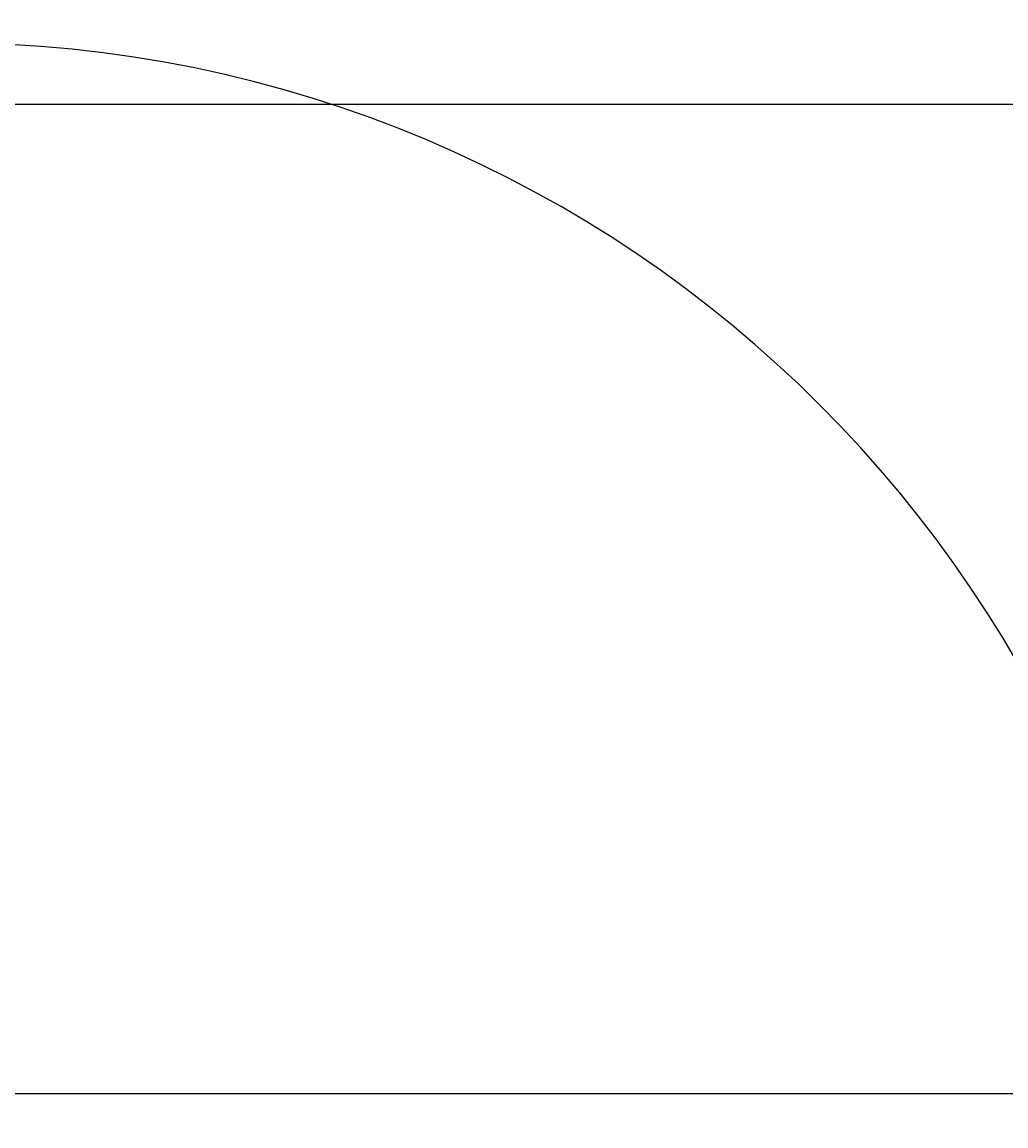
# Model space of a CAD drawing. Units: inches. Extents: x 2231 to 2461, y 2045 to 2455.
# Tile 6 of 95: x 2303 to 2326, y 2072 to 2099. Entities that reach past the tile are written whole.
import ezdxf

# ---------------------------------------------------------------- set-up
doc = ezdxf.new("R2010")
doc.units = ezdxf.units.IN
doc.layers.add('A-ANNO-DIMS', color=2, linetype='Continuous', lineweight=18)
doc.layers.add('A-DOOR', color=3, linetype='Continuous', lineweight=25)
doc.styles.get("Standard").update_dxf_attribs({"font": 'arial.ttf'})
doc.dimstyles.get("Standard").update_dxf_attribs({"dimtxt": 0.18, "dimasz": 0.18, "dimexe": 0.18, "dimexo": 0.0625, "dimgap": 0.09, "dimtad": 0, "dimtih": 1, "dimtoh": 1, "dimdec": 4, "dimzin": 0, "dimdsep": 46, "dimtxsty": 'Standard', "dimcen": 0.09, "dimadec": 0, "dimazin": 0, "dimtfac": 1, "dimtdec": 4, "dimtofl": 0, "dimtmove": 0, "dimatfit": 3, "dimfxl": 1, "dimtolj": 1, "dimtzin": 0, "dimarcsym": 0})

# ---------------------------------------------------------------- blocks, each defined once
blk = doc.blocks.new('*U5')
blk.add_arc((0, 0), 40, 0, 90)
blk = doc.blocks.new('*D51')
at = {"layer": 'A-ANNO-DIMS', "color": 0, "lineweight": -2, "transparency": 16777216}
for p, q in [((2258.794, 2306.77), (2258.794, 2044.803)), ((2330.794, 2306.77), (2330.794, 2044.803)), ((2258.974, 2044.983), (2294.576, 2044.983)), ((2330.614, 2044.983), (2295.011, 2044.983))]:
    blk.add_line(p, q, dxfattribs=at)
at = {"layer": 'A-ANNO-DIMS', "color": 0, "transparency": 16777216}
for points in [[(2258.974, 2045.013), (2258.974, 2044.953), (2258.794, 2044.983)], [(2330.614, 2045.013), (2330.614, 2044.953), (2330.794, 2044.983)]]:
    blk.add_solid(points, dxfattribs=at)
at = {"layer": 'Defpoints', "color": 0, "transparency": 16777216}
for p in [(2258.794, 2306.833), (2330.794, 2306.833), (2330.794, 2044.983)]:
    blk.add_point(p, dxfattribs=at)
at = {"layer": 'A-ANNO-DIMS', "color": 0, "transparency": 16777216, "insert": (2294.794, 2044.983), "char_height": 0.18, "attachment_point": 5}
blk.add_mtext('\\A1;72', dxfattribs=at)
blk = doc.blocks.new('*D65')
at = {"layer": 'A-ANNO-DIMS', "color": 0, "lineweight": -2, "transparency": 16777216}
for p, q in [((2285.635, 2189.285), (2285.635, 2044.803)), ((2340.667, 2189.285), (2340.667, 2044.803)), ((2285.815, 2044.983), (2312.758, 2044.983)), ((2340.487, 2044.983), (2313.545, 2044.983))]:
    blk.add_line(p, q, dxfattribs=at)
at = {"layer": 'A-ANNO-DIMS', "color": 0, "transparency": 16777216}
for points in [[(2285.815, 2045.013), (2285.815, 2044.953), (2285.635, 2044.983)], [(2340.487, 2045.013), (2340.487, 2044.953), (2340.667, 2044.983)]]:
    blk.add_solid(points, dxfattribs=at)
at = {"layer": 'Defpoints', "color": 0, "transparency": 16777216}
for p in [(2285.635, 2189.348), (2340.667, 2189.348), (2340.667, 2044.983)]:
    blk.add_point(p, dxfattribs=at)
at = {"layer": 'A-ANNO-DIMS', "color": 0, "transparency": 16777216, "insert": (2313.151, 2044.983), "char_height": 0.18, "attachment_point": 5}
blk.add_mtext('\\A1;55.03', dxfattribs=at)
blk = doc.blocks.new('*D67')
at = {"layer": 'A-ANNO-DIMS', "color": 0, "lineweight": -2, "transparency": 16777216}
for p, q in [((2348.126, 2096.833), (2230.981, 2096.833)), ((2231.161, 2096.653), (2231.161, 2085.013)), ((2231.161, 2073.013), (2231.161, 2084.652)), ((2348.559, 2072.833), (2230.981, 2072.833))]:
    blk.add_line(p, q, dxfattribs=at)
at = {"layer": 'A-ANNO-DIMS', "color": 0, "transparency": 16777216}
for points in [[(2231.131, 2096.653), (2231.191, 2096.653), (2231.161, 2096.833)], [(2231.131, 2073.013), (2231.191, 2073.013), (2231.161, 2072.833)]]:
    blk.add_solid(points, dxfattribs=at)
at = {"layer": 'Defpoints', "color": 0, "transparency": 16777216}
for p in [(2348.189, 2096.833), (2231.161, 2072.833), (2348.622, 2072.833)]:
    blk.add_point(p, dxfattribs=at)
at = {"layer": 'A-ANNO-DIMS', "color": 0, "transparency": 16777216, "insert": (2231.161, 2084.833), "char_height": 0.18, "attachment_point": 5}
blk.add_mtext('\\A1;24', dxfattribs=at)

msp = doc.modelspace()

# ---------------------------------------------------------------- block references
at = {"layer": 'A-DOOR', "xscale": 0.75, "yscale": 0.75, "zscale": 0.75}
msp.add_blockref('*U5', (2300.7392, 2068.3328), dxfattribs=at)

# ---------------------------------------------------------------- dimensions: what is measured, and where the dimension line sits
at = {"layer": 'A-ANNO-DIMS'}
for base, p1, p2, override, picture, middle in [((2330.7935, 2044.9825), (2258.7935, 2306.8328), (2330.7935, 2306.8328), {"dimdec": 0, "dimlfac": 1, "dimrnd": 0, "dimzin": 0, "dimdsep": 46, "dimlunit": 2}, '*D51', (2294.7935, 2044.9825)), ((2340.6673, 2044.9825), (2285.6353, 2189.3477), (2340.6673, 2189.3477), {"dimdec": 2, "dimlfac": 1, "dimrnd": 0, "dimzin": 0, "dimdsep": 46, "dimlunit": 2}, '*D65', (2313.1513, 2044.9825))]:
    dim = msp.add_linear_dim(base=base, p1=p1, p2=p2, dimstyle='Standard', override=override, dxfattribs=at)
    dim.commit()
    dim.dimension.update_dxf_attribs({"geometry": picture, "text_midpoint": middle})
dim = msp.add_linear_dim(base=(2231.161, 2072.8328), p1=(2348.1888, 2096.8328), p2=(2348.6219, 2072.8328), angle=90, dimstyle='Standard', override={"dimdec": 0, "dimlfac": 1, "dimrnd": 0, "dimzin": 0, "dimdsep": 46, "dimlunit": 2}, dxfattribs=at)
dim.commit()
dim.dimension.update_dxf_attribs({"geometry": '*D67', "text_midpoint": (2231.161, 2084.8328)})

doc.saveas('drawing.dxf')
